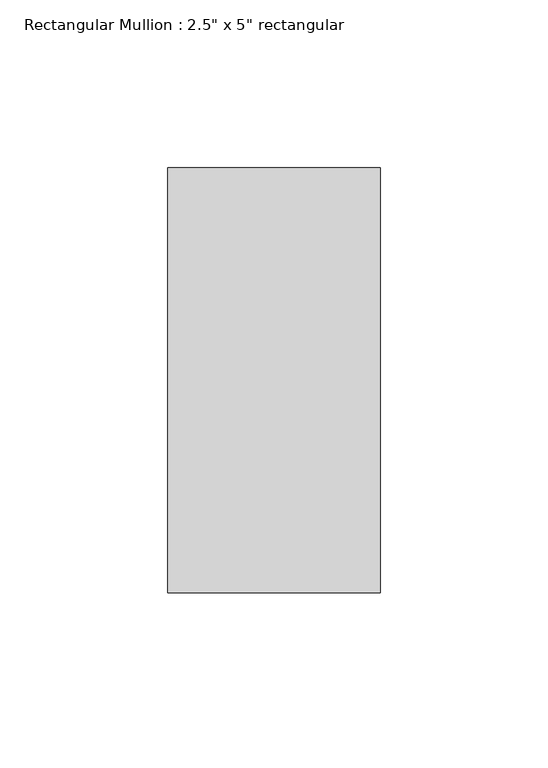
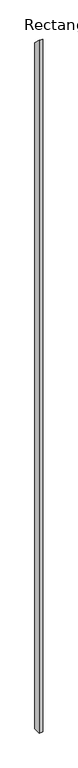
"""IFC4 building model written with IfcOpenShell, lengths in millimetres: member geometry."""

from ifc_helpers import new_model, si_unit, frame, origin, place, context, project, spatial, polyline, outline, extrude, source, transform, mapped, element, save


def member_0d72fb60(model_context):
    return source(origin(), model_context, "Body", "SweptSolid", [
        extrude(outline(polyline([(-63.5, 63.5), (63.5, -63.5), (63.5, -12738.978371), (-63.5, -12738.978371), (-63.5, 63.5)])), frame((-63.5, 0.0, 0.0), z_axis=(1.0, 0.0, 0.0), x_axis=(0.0, 1.0, 0.0)), (0.0, 0.0, 1.0), 63.5),
    ])


if __name__ == "__main__":
    model = new_model("IFC4")
    model_context = context("Model", 3, world=origin())
    ifc_project = project(units=[si_unit("LENGTHUNIT", "METRE", prefix="MILLI")], contexts=[model_context])
    site = spatial("IfcSite", under=ifc_project)
    building = spatial("IfcBuilding", under=site)
    placement = place(None, origin())
    member_shape = member_0d72fb60(model_context)
    element("IfcMember", 1, ObjectType="Rectangular Mullion : 2.5\" x 5\" rectangular", at=placement, inside=building, context=model_context, shape_type="MappedRepresentation", body=[
        mapped(member_shape, transform((0.0, 0.0, 0.0), x_axis=(1.0, 0.0, 0.0), y_axis=(0.0, 1.0, 0.0), z_axis=(0.0, 0.0, 1.0))),
    ])
    save(model, "model.ifc")

# Revit data of these elements
# Type "Rectangular Mullion : 2.5\" x 5\" rectangular"
#   built-in parameter 1007304 = 0.416667 (stored number, unit not read)
#   built-in parameter 1007301 = 0.104167 (stored number, unit not read)
#   built-in parameter 1007300 = 0.104167 (stored number, unit not read)
# Element 1 (IfcMember, "Rectangular Mullion : 2.5\" x 5\" rectangular")
#   Materials on its faces: "Aluminum"
# Materials
#   "Aluminum": class "Metal", colour RGB 247 247 247, transparency 0, Description = "Aluminum 6061", Cost = 0
